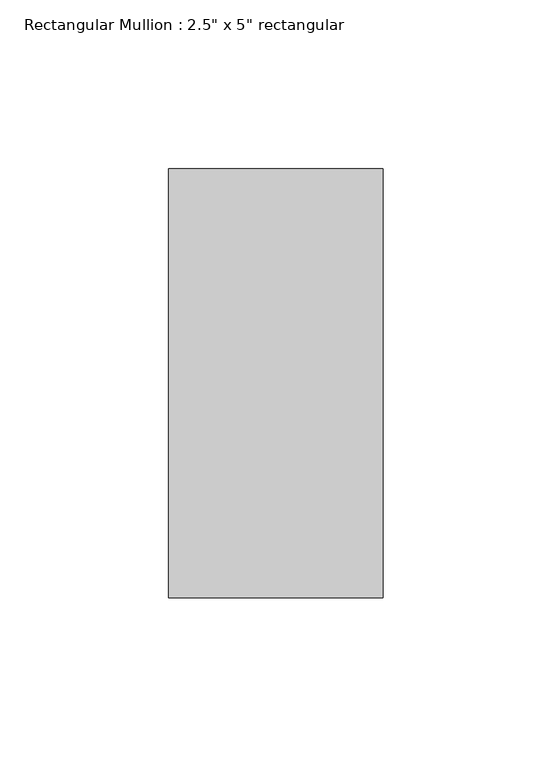
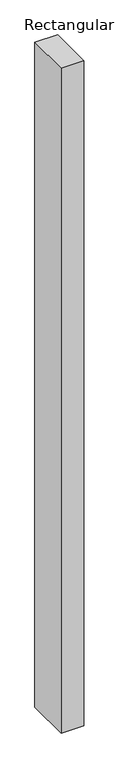
"""IFC4 building model written with IfcOpenShell, lengths in millimetres: member geometry."""

from ifc_helpers import new_model, si_unit, frame, origin, place, context, project, spatial, polyline, outline, extrude, source, transform, mapped, element, save


def member_0bd10330(model_context):
    return source(origin(), model_context, "Body", "SweptSolid", [
        extrude(outline(polyline([(0.0, 63.5), (0.0, -63.5), (-63.5, -63.5), (-63.5, 63.5), (0.0, 63.5)])), frame((0.0, 0.0, -1964.4891744), z_axis=(0.0, 0.0, 1.0), x_axis=(1.0, 0.0, 0.0)), (0.0, 0.0, 1.0), 1964.4891744),
    ])


if __name__ == "__main__":
    model = new_model("IFC4")
    model_context = context("Model", 3, world=origin())
    ifc_project = project(units=[si_unit("LENGTHUNIT", "METRE", prefix="MILLI")], contexts=[model_context])
    site = spatial("IfcSite", under=ifc_project)
    building = spatial("IfcBuilding", under=site)
    placement = place(None, origin())
    member_shape = member_0bd10330(model_context)
    element("IfcMember", 1, ObjectType="Rectangular Mullion : 2.5\" x 5\" rectangular", at=placement, inside=building, context=model_context, shape_type="MappedRepresentation", body=[
        mapped(member_shape, transform((0.0, 0.0, 0.0), x_axis=(1.0, 0.0, 0.0), y_axis=(0.0, 1.0, 0.0), z_axis=(0.0, 0.0, 1.0))),
    ])
    save(model, "model.ifc")

# Revit data of these elements
# Type "Rectangular Mullion : 2.5\" x 5\" rectangular"
#   built-in parameter 1007304 = 0.416667 (stored number, unit not read)
#   built-in parameter 1007301 = 0.104167 (stored number, unit not read)
#   built-in parameter 1007300 = 0.104167 (stored number, unit not read)
# Element 1 (IfcMember, "Rectangular Mullion : 2.5\" x 5\" rectangular")
#   Materials on its faces: "Aluminum"
# Materials
#   "Aluminum": class "Metal", colour RGB 247 247 247, transparency 0, Description = "Aluminum 6061", Cost = 0
